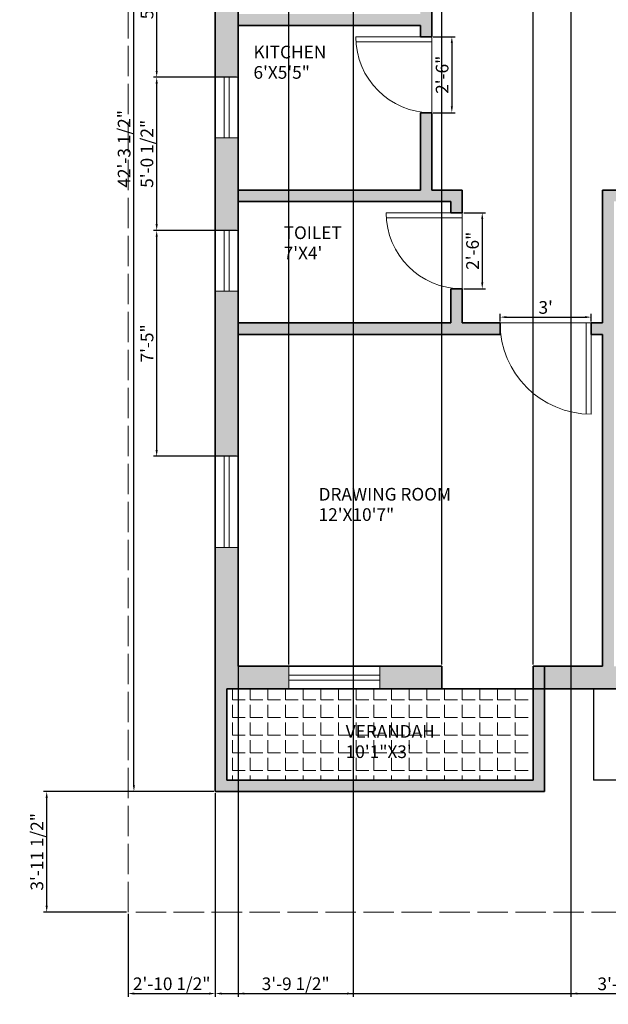
# Model space of a CAD drawing. Units: inches. Extents: x 2871 to 3419, y 1549 to 2228.
# Tile 1 of 3: x 2871 to 3103, y 1549 to 1938. Entities that reach past the tile are written whole.
import ezdxf

# ---------------------------------------------------------------- set-up
doc = ezdxf.new("R2010")
doc.units = ezdxf.units.IN
doc.linetypes.add('ACAD_ISO02W100', pattern=[15, 12, -3])
for name, color, linetype, lineweight in [('A-ANNO-DIMS', 3, 'Continuous', 13), ('A-AREA-IDEN', 3, 'Continuous', 18), ('A-FLOR', 7, 'Continuous', 25), ('A-FLOR-PATT', 30, 'Continuous', 13), ('A-WALL-PATT', 18, 'Continuous', 13), ('C-PROP', 7, 'ACAD_ISO02W100', 18), ('doors', 6, 'Continuous', 18), ('wall', 4, 'Continuous', 35), ('windows', 1, 'Continuous', 18)]:
    doc.layers.add(name, color=color, linetype=linetype, lineweight=lineweight)
doc.styles.get("Standard").update_dxf_attribs({"font": 'arial.ttf', "height": 5})
doc.dimstyles.new('ISO-25', dxfattribs={"dimtxt": 5, "dimasz": 2.5, "dimexe": 1.25, "dimexo": 0.625, "dimtad": 1, "dimlunit": 3, "dimtxsty": 'Standard', "dimcen": 2.5, "dimadec": 0, "dimazin": 0, "dimtfac": 1, "dimtmove": 0, "dimatfit": 3, "dimfxl": 1, "dimarcsym": 0})

# ---------------------------------------------------------------- blocks, each defined once
blk = doc.blocks.new('*D9')
at = {"layer": 'A-ANNO-DIMS', "color": 0, "lineweight": -2, "transparency": 16777216}
for p, q in [((3060.42, 1818.86), (3060.42, 1821.79)), ((3062.92, 1820.54), (3093.92, 1820.54)), ((3096.42, 1818.86), (3096.42, 1821.79))]:
    blk.add_line(p, q, dxfattribs=at)
at = {"layer": 'A-ANNO-DIMS', "color": 0, "transparency": 16777216}
for points in [[(3062.92, 1820.96), (3062.92, 1820.13), (3060.42, 1820.54)], [(3093.92, 1820.96), (3093.92, 1820.13), (3096.42, 1820.54)]]:
    blk.add_solid(points, dxfattribs=at)
at = {"layer": 'Defpoints', "color": 0, "transparency": 16777216}
for p in [(3096.42, 1820.54), (3060.42, 1818.24), (3096.42, 1818.24)]:
    blk.add_point(p, dxfattribs=at)
at = {"layer": 'A-ANNO-DIMS', "color": 0, "transparency": 16777216, "insert": (3078.42, 1823.72), "char_height": 5, "attachment_point": 5}
blk.add_mtext("3'", dxfattribs=at)
blk = doc.blocks.new('*D10')
at = {"layer": 'A-ANNO-DIMS', "color": 0, "lineweight": -2, "transparency": 16777216}
for p, q in [((3046.04, 1861.74), (3054.62, 1861.74)), ((3053.37, 1859.24), (3053.37, 1834.24)), ((3046.04, 1831.74), (3054.62, 1831.74))]:
    blk.add_line(p, q, dxfattribs=at)
at = {"layer": 'A-ANNO-DIMS', "color": 0, "transparency": 16777216}
for points in [[(3052.95, 1859.24), (3053.79, 1859.24), (3053.37, 1861.74)], [(3052.95, 1834.24), (3053.79, 1834.24), (3053.37, 1831.74)]]:
    blk.add_solid(points, dxfattribs=at)
at = {"layer": 'Defpoints', "color": 0, "transparency": 16777216}
for p in [(3045.42, 1861.74), (3045.42, 1831.74), (3053.37, 1831.74)]:
    blk.add_point(p, dxfattribs=at)
at = {"layer": 'A-ANNO-DIMS', "color": 0, "transparency": 16777216, "insert": (3050.19, 1846.74), "char_height": 5, "attachment_point": 5, "rotation": 90}
blk.add_mtext('2\'-6"', dxfattribs=at)
blk = doc.blocks.new('*D11')
at = {"layer": 'A-ANNO-DIMS', "color": 0, "lineweight": -2, "transparency": 16777216}
for p, q in [((3034.04, 1931.24), (3042.61, 1931.24)), ((3041.36, 1928.74), (3041.36, 1903.74)), ((3034.04, 1901.24), (3042.61, 1901.24))]:
    blk.add_line(p, q, dxfattribs=at)
at = {"layer": 'A-ANNO-DIMS', "color": 0, "transparency": 16777216}
for points in [[(3040.94, 1928.74), (3041.77, 1928.74), (3041.36, 1931.24)], [(3040.94, 1903.74), (3041.77, 1903.74), (3041.36, 1901.24)]]:
    blk.add_solid(points, dxfattribs=at)
at = {"layer": 'Defpoints', "color": 0, "transparency": 16777216}
for p in [(3033.42, 1931.24), (3033.42, 1901.24), (3041.36, 1901.24)]:
    blk.add_point(p, dxfattribs=at)
at = {"layer": 'A-ANNO-DIMS', "color": 0, "transparency": 16777216, "insert": (3038.18, 1916.24), "char_height": 5, "attachment_point": 5, "rotation": 90}
blk.add_mtext('2\'-6"', dxfattribs=at)
blk = doc.blocks.new('WIN-36IN')
for p, q in [((0, 36), (0, 0)), ((9, 36), (0, 36)), ((3.5, 0), (3.5, 36)), ((5.5, 0), (5.5, 36)), ((9, 0), (9, 36)), ((0, 0), (9, 0))]:
    blk.add_line(p, q)
blk = doc.blocks.new('WIN-24IN')
for p, q in [((0, 24), (0, 0)), ((9, 24), (0, 24)), ((3.5, 0), (3.5, 24)), ((5.5, 0), (5.5, 24)), ((9, 0), (9, 24)), ((0, 0), (9, 0))]:
    blk.add_line(p, q)
blk = doc.blocks.new('DOOR-SWING-30IN')
for p, q in [((28, 29.93), (28, 0)), ((30, 30), (30, 0)), ((30, 0), (0, 0))]:
    blk.add_line(p, q)
blk.add_arc((30, 0), 30, 90, 180)
blk = doc.blocks.new('DOOR-SWING-36IN')
for p, q in [((0, 36), (0, 0)), ((2, 35.94), (2, 0)), ((0, 0), (36, 0))]:
    blk.add_line(p, q)
blk.add_arc((0, 0), 36, 0, 90)
blk = doc.blocks.new('*D22')
at = {"layer": 'A-ANNO-DIMS', "color": 0, "lineweight": -2, "transparency": 16777216}
for p, q in [((2947.92, 1632.61), (2947.92, 1552.22)), ((3349.42, 1632.61), (3349.42, 1552.22)), ((2950.42, 1553.47), (3346.92, 1553.47))]:
    blk.add_line(p, q, dxfattribs=at)
at = {"layer": 'A-ANNO-DIMS', "color": 0, "transparency": 16777216}
for points in [[(2950.42, 1553.89), (2950.42, 1553.05), (2947.92, 1553.47)], [(3346.92, 1553.89), (3346.92, 1553.05), (3349.42, 1553.47)]]:
    blk.add_solid(points, dxfattribs=at)
at = {"layer": 'Defpoints', "color": 0, "transparency": 16777216}
for p in [(2947.92, 1633.24), (3349.42, 1633.24), (3349.42, 1553.47)]:
    blk.add_point(p, dxfattribs=at)
at = {"layer": 'A-ANNO-DIMS', "color": 0, "transparency": 16777216, "insert": (3148.67, 1556.68), "char_height": 5, "attachment_point": 5}
blk.add_mtext('33\'-5 1/2"', dxfattribs=at)
blk = doc.blocks.new('*D23')
at = {"layer": 'A-ANNO-DIMS', "color": 0, "lineweight": -2, "transparency": 16777216}
for p, q in [((2947.29, 2140.74), (2914.52, 2140.74)), ((2915.77, 1635.74), (2915.77, 2138.24)), ((2947.29, 1633.24), (2914.52, 1633.24))]:
    blk.add_line(p, q, dxfattribs=at)
at = {"layer": 'A-ANNO-DIMS', "color": 0, "transparency": 16777216}
for points in [[(2915.35, 2138.24), (2916.18, 2138.24), (2915.77, 2140.74)], [(2915.35, 1635.74), (2916.18, 1635.74), (2915.77, 1633.24)]]:
    blk.add_solid(points, dxfattribs=at)
at = {"layer": 'Defpoints', "color": 0, "transparency": 16777216}
for p in [(2915.77, 2140.74), (2947.92, 2140.74), (2947.92, 1633.24)]:
    blk.add_point(p, dxfattribs=at)
at = {"layer": 'A-ANNO-DIMS', "color": 0, "transparency": 16777216, "insert": (2912.56, 1886.99), "char_height": 5, "attachment_point": 5, "rotation": 90}
blk.add_mtext('42\'-3 1/2"', dxfattribs=at)
blk = doc.blocks.new('*D24')
at = {"layer": 'A-ANNO-DIMS', "color": 0, "lineweight": -2, "transparency": 16777216}
for p, q in [((2947.92, 1632.61), (2947.92, 1552.22)), ((2913.47, 1585), (2913.47, 1552.22)), ((2915.97, 1553.47), (2945.42, 1553.47))]:
    blk.add_line(p, q, dxfattribs=at)
at = {"layer": 'A-ANNO-DIMS', "color": 0, "transparency": 16777216}
for points in [[(2915.97, 1553.89), (2915.97, 1553.05), (2913.47, 1553.47)], [(2945.42, 1553.89), (2945.42, 1553.05), (2947.92, 1553.47)]]:
    blk.add_solid(points, dxfattribs=at)
at = {"layer": 'Defpoints', "color": 0, "transparency": 16777216}
for p in [(2947.92, 1633.24), (2913.47, 1585.62), (2947.92, 1553.47)]:
    blk.add_point(p, dxfattribs=at)
at = {"layer": 'A-ANNO-DIMS', "color": 0, "transparency": 16777216, "insert": (2930.69, 1556.68), "char_height": 5, "attachment_point": 5}
blk.add_mtext('2\'-10 1/2"', dxfattribs=at)
blk = doc.blocks.new('*D25')
at = {"layer": 'A-ANNO-DIMS', "color": 0, "lineweight": -2, "transparency": 16777216}
for p, q in [((2947.29, 1633.24), (2880.07, 1633.24)), ((2881.32, 1588.12), (2881.32, 1630.74)), ((2912.84, 1585.62), (2880.07, 1585.62))]:
    blk.add_line(p, q, dxfattribs=at)
at = {"layer": 'A-ANNO-DIMS', "color": 0, "transparency": 16777216}
for points in [[(2880.9, 1630.74), (2881.73, 1630.74), (2881.32, 1633.24)], [(2880.9, 1588.12), (2881.73, 1588.12), (2881.32, 1585.62)]]:
    blk.add_solid(points, dxfattribs=at)
at = {"layer": 'Defpoints', "color": 0, "transparency": 16777216}
for p in [(2881.32, 1633.24), (2947.92, 1633.24), (2913.47, 1585.62)]:
    blk.add_point(p, dxfattribs=at)
at = {"layer": 'A-ANNO-DIMS', "color": 0, "transparency": 16777216, "insert": (2878.11, 1609.43), "char_height": 5, "attachment_point": 5, "rotation": 90}
blk.add_mtext('3\'-11 1/2"', dxfattribs=at)
blk = doc.blocks.new('*D26')
at = {"layer": 'A-ANNO-DIMS', "color": 0, "lineweight": -2, "transparency": 16777216}
for p, q in [((2956.92, 2131.11), (2956.92, 1552.22)), ((3002.42, 2131.11), (3002.42, 1552.22)), ((2959.42, 1553.47), (2999.92, 1553.47))]:
    blk.add_line(p, q, dxfattribs=at)
at = {"layer": 'A-ANNO-DIMS', "color": 0, "transparency": 16777216}
for points in [[(2959.42, 1553.89), (2959.42, 1553.05), (2956.92, 1553.47)], [(2999.92, 1553.89), (2999.92, 1553.05), (3002.42, 1553.47)]]:
    blk.add_solid(points, dxfattribs=at)
at = {"layer": 'Defpoints', "color": 0, "transparency": 16777216}
for p in [(2956.92, 2131.74), (3002.42, 2131.74), (3002.42, 1553.47)]:
    blk.add_point(p, dxfattribs=at)
at = {"layer": 'A-ANNO-DIMS', "color": 0, "transparency": 16777216, "insert": (2979.67, 1556.68), "char_height": 5, "attachment_point": 5}
blk.add_mtext('3\'-9 1/2"', dxfattribs=at)
blk = doc.blocks.new('*D27')
at = {"layer": 'A-ANNO-DIMS', "color": 0, "lineweight": -2, "transparency": 16777216}
for p, q in [((3088.42, 2131.11), (3088.42, 1552.22)), ((3124.42, 2131.11), (3124.42, 1552.22)), ((3090.92, 1553.47), (3121.92, 1553.47))]:
    blk.add_line(p, q, dxfattribs=at)
at = {"layer": 'A-ANNO-DIMS', "color": 0, "transparency": 16777216}
for points in [[(3090.92, 1553.89), (3090.92, 1553.05), (3088.42, 1553.47)], [(3121.92, 1553.89), (3121.92, 1553.05), (3124.42, 1553.47)]]:
    blk.add_solid(points, dxfattribs=at)
at = {"layer": 'Defpoints', "color": 0, "transparency": 16777216}
for p in [(3088.42, 2131.74), (3124.42, 2131.74), (3124.42, 1553.47)]:
    blk.add_point(p, dxfattribs=at)
at = {"layer": 'A-ANNO-DIMS', "color": 0, "transparency": 16777216, "insert": (3106.42, 1556.65), "char_height": 5, "attachment_point": 5}
blk.add_mtext('3\'-0"', dxfattribs=at)
blk = doc.blocks.new('*D41')
at = {"layer": 'A-ANNO-DIMS', "color": 0, "lineweight": -2, "transparency": 16777216}
for p, q in [((2956.29, 1976.06), (2923.52, 1976.06)), ((2924.77, 1917.79), (2924.77, 1973.56)), ((2956.29, 1915.29), (2923.52, 1915.29))]:
    blk.add_line(p, q, dxfattribs=at)
at = {"layer": 'A-ANNO-DIMS', "color": 0, "transparency": 16777216}
for points in [[(2924.35, 1973.56), (2925.18, 1973.56), (2924.77, 1976.06)], [(2924.35, 1917.79), (2925.18, 1917.79), (2924.77, 1915.29)]]:
    blk.add_solid(points, dxfattribs=at)
at = {"layer": 'Defpoints', "color": 0, "transparency": 16777216}
for p in [(2924.77, 1976.06), (2956.92, 1976.06), (2956.92, 1915.29)]:
    blk.add_point(p, dxfattribs=at)
at = {"layer": 'A-ANNO-DIMS', "color": 0, "transparency": 16777216, "insert": (2921.59, 1945.68), "char_height": 5, "attachment_point": 5, "rotation": 90}
blk.add_mtext('5\'-1"', dxfattribs=at)
blk = doc.blocks.new('*D42')
at = {"layer": 'A-ANNO-DIMS', "color": 0, "lineweight": -2, "transparency": 16777216}
for p, q in [((2956.29, 1915.29), (2923.52, 1915.29)), ((2924.77, 1857.27), (2924.77, 1912.79)), ((2956.29, 1854.77), (2923.52, 1854.77))]:
    blk.add_line(p, q, dxfattribs=at)
at = {"layer": 'A-ANNO-DIMS', "color": 0, "transparency": 16777216}
for points in [[(2924.35, 1912.79), (2925.18, 1912.79), (2924.77, 1915.29)], [(2924.35, 1857.27), (2925.18, 1857.27), (2924.77, 1854.77)]]:
    blk.add_solid(points, dxfattribs=at)
at = {"layer": 'Defpoints', "color": 0, "transparency": 16777216}
for p in [(2924.77, 1915.29), (2956.92, 1915.29), (2956.92, 1854.77)]:
    blk.add_point(p, dxfattribs=at)
at = {"layer": 'A-ANNO-DIMS', "color": 0, "transparency": 16777216, "insert": (2921.56, 1885.03), "char_height": 5, "attachment_point": 5, "rotation": 90}
blk.add_mtext('5\'-0 1/2"', dxfattribs=at)
blk = doc.blocks.new('*D43')
at = {"layer": 'A-ANNO-DIMS', "color": 0, "lineweight": -2, "transparency": 16777216}
for p, q in [((2956.29, 1854.77), (2923.52, 1854.77)), ((2924.77, 1768.09), (2924.77, 1852.27)), ((2956.29, 1765.59), (2923.52, 1765.59))]:
    blk.add_line(p, q, dxfattribs=at)
at = {"layer": 'A-ANNO-DIMS', "color": 0, "transparency": 16777216}
for points in [[(2924.35, 1852.27), (2925.18, 1852.27), (2924.77, 1854.77)], [(2924.35, 1768.09), (2925.18, 1768.09), (2924.77, 1765.59)]]:
    blk.add_solid(points, dxfattribs=at)
at = {"layer": 'Defpoints', "color": 0, "transparency": 16777216}
for p in [(2924.77, 1854.77), (2956.92, 1854.77), (2956.92, 1765.59)]:
    blk.add_point(p, dxfattribs=at)
at = {"layer": 'A-ANNO-DIMS', "color": 0, "transparency": 16777216, "insert": (2921.6, 1810.18), "char_height": 5, "attachment_point": 5, "rotation": 90}
blk.add_mtext('7\'-5"', dxfattribs=at)
blk = doc.blocks.new('*D44')
at = {"layer": 'A-ANNO-DIMS', "color": 0, "lineweight": -2, "transparency": 16777216}
for p, q in [((2956.92, 1683.36), (2956.92, 2219.02)), ((2959.42, 2217.77), (2974.42, 2217.77)), ((2976.92, 1683.36), (2976.92, 2219.02))]:
    blk.add_line(p, q, dxfattribs=at)
at = {"layer": 'A-ANNO-DIMS', "color": 0, "transparency": 16777216}
for points in [[(2959.42, 2218.19), (2959.42, 2217.35), (2956.92, 2217.77)], [(2974.42, 2218.19), (2974.42, 2217.35), (2976.92, 2217.77)]]:
    blk.add_solid(points, dxfattribs=at)
at = {"layer": 'Defpoints', "color": 0, "transparency": 16777216}
for p in [(2976.92, 2217.77), (2956.92, 1682.74), (2976.92, 1682.74)]:
    blk.add_point(p, dxfattribs=at)
at = {"layer": 'A-ANNO-DIMS', "color": 0, "transparency": 16777216, "insert": (2966.92, 2220.95), "char_height": 5, "attachment_point": 5}
blk.add_mtext('1\'-8"', dxfattribs=at)
blk = doc.blocks.new('*D46')
at = {"layer": 'A-ANNO-DIMS', "color": 0, "lineweight": -2, "transparency": 16777216}
for p, q in [((3037.42, 1683.36), (3037.42, 2219.02)), ((3039.92, 2217.77), (3070.92, 2217.77)), ((3073.42, 1683.36), (3073.42, 2219.02))]:
    blk.add_line(p, q, dxfattribs=at)
at = {"layer": 'A-ANNO-DIMS', "color": 0, "transparency": 16777216}
for points in [[(3039.92, 2218.19), (3039.92, 2217.35), (3037.42, 2217.77)], [(3070.92, 2218.19), (3070.92, 2217.35), (3073.42, 2217.77)]]:
    blk.add_solid(points, dxfattribs=at)
at = {"layer": 'Defpoints', "color": 0, "transparency": 16777216}
for p in [(3073.42, 2217.77), (3037.42, 1682.74), (3073.42, 1682.74)]:
    blk.add_point(p, dxfattribs=at)
at = {"layer": 'A-ANNO-DIMS', "color": 0, "transparency": 16777216, "insert": (3055.42, 2220.95), "char_height": 5, "attachment_point": 5}
blk.add_mtext('3\'-0"', dxfattribs=at)
blk = doc.blocks.new('*D48')
at = {"layer": 'A-ANNO-DIMS', "color": 0, "lineweight": -2, "transparency": 16777216}
for p, q in [((2976.92, 1683.36), (2976.92, 2219.02)), ((2979.42, 2217.77), (3034.92, 2217.77)), ((3037.42, 1683.36), (3037.42, 2219.02))]:
    blk.add_line(p, q, dxfattribs=at)
at = {"layer": 'A-ANNO-DIMS', "color": 0, "transparency": 16777216}
for points in [[(2979.42, 2218.19), (2979.42, 2217.35), (2976.92, 2217.77)], [(3034.92, 2218.19), (3034.92, 2217.35), (3037.42, 2217.77)]]:
    blk.add_solid(points, dxfattribs=at)
at = {"layer": 'Defpoints', "color": 0, "transparency": 16777216}
for p in [(3037.42, 2217.77), (2976.92, 1682.74), (3037.42, 1682.74)]:
    blk.add_point(p, dxfattribs=at)
at = {"layer": 'A-ANNO-DIMS', "color": 0, "transparency": 16777216, "insert": (3007.17, 2220.98), "char_height": 5, "attachment_point": 5}
blk.add_mtext('5\'-0 1/2"', dxfattribs=at)

msp = doc.modelspace()

# ---------------------------------------------------------------- hatches: boundary and pattern name
at = {"layer": 'A-FLOR-PATT'}
h = msp.add_hatch(dxfattribs=at)
h.set_pattern_fill('ANGLE', color=256)
h.set_pattern_definition([(0, (0, 0), (0, 6.985), [5.08, -1.905]), (90, (0, 0), (-6.985, 4e-16), [5.08, -1.905])])
h.paths.add_polyline_path([(3073.418, 1673.735), (3037.418, 1673.735), (2952.418, 1673.735), (2952.418, 1637.735), (3073.418, 1637.735)])
h.paths.add_polyline_path([(3344.918, 1673.735), (3259.918, 1673.735), (3223.918, 1673.735), (3223.918, 1637.735), (3344.918, 1637.735)])
h.paths.add_polyline_path([(2998.155, 1645.095), (3026.055, 1645.095), (3026.055, 1652.758), (2998.155, 1652.758)], flags=24)
h.paths.add_polyline_path([(2998.183, 1653.243), (3039.496, 1653.243), (3039.496, 1660.743), (2998.183, 1660.743)], flags=24)
h.paths.add_polyline_path([(3263.884, 1645.095), (3291.783, 1645.095), (3291.783, 1652.758), (3263.884, 1652.758)], flags=24)
h.paths.add_polyline_path([(3263.911, 1653.243), (3305.224, 1653.243), (3305.224, 1660.743), (3263.911, 1660.743)], flags=24)
at = {"layer": 'A-WALL-PATT'}
h = msp.add_hatch(color=256, dxfattribs=at)
h.dxf.hatch_style = 1
h.paths.add_polyline_path([(2956.918, 2131.735), (3002.418, 2131.735), (3002.418, 2140.735), (2947.918, 2140.735), (2947.918, 2079.154), (2956.918, 2079.154)])
h.paths.add_polyline_path([(3252.668, 2140.735), (3160.418, 2140.735), (3160.418, 2131.735), (3196.418, 2131.735), (3196.418, 1992.735), (3128.918, 1992.735), (3128.918, 1988.235), (3160.418, 1988.235), (3160.418, 1870.735), (3160.418, 1866.235), (3164.918, 1866.235), (3164.918, 1890.235), (3164.918, 1988.235), (3205.418, 1988.235), (3205.418, 1992.735), (3200.918, 1992.735), (3200.918, 2131.735), (3252.668, 2131.735)])
h.paths.add_polyline_path([(3349.418, 2140.735), (3288.668, 2140.735), (3288.668, 2131.735), (3340.418, 2131.735), (3340.418, 2080.235), (3349.418, 2080.235)])
h.paths.add_polyline_path([(3349.418, 2044.235), (3340.418, 2044.235), (3340.418, 1992.735), (3302.918, 1992.735), (3302.918, 1988.235), (3340.418, 1988.235), (3340.418, 1976.235), (3349.418, 1976.235)])
h.paths.add_polyline_path([(3349.418, 1952.235), (3340.418, 1952.235), (3340.418, 1940.235), (3268.418, 1940.235), (3268.418, 1988.235), (3272.918, 1988.235), (3272.918, 1992.735), (3241.418, 1992.735), (3241.418, 1988.235), (3263.918, 1988.235), (3263.918, 1931.235), (3268.418, 1931.235), (3268.418, 1935.735), (3340.418, 1935.735), (3340.418, 1915.235), (3349.418, 1915.235)])
h.paths.add_polyline_path([(3349.418, 1891.235), (3340.418, 1891.235), (3340.418, 1870.735), (3268.418, 1870.735), (3268.418, 1901.235), (3263.918, 1901.235), (3263.918, 1870.735), (3251.918, 1870.735), (3251.918, 1866.235), (3251.918, 1861.735), (3256.418, 1861.735), (3256.418, 1866.235), (3340.418, 1866.235), (3340.418, 1854.235), (3349.418, 1854.235)])
h.paths.add_polyline_path([(3349.418, 1830.235), (3340.418, 1830.235), (3340.418, 1818.235), (3256.418, 1818.235), (3256.418, 1831.735), (3251.918, 1831.735), (3251.918, 1818.235), (3236.918, 1818.235), (3236.918, 1813.735), (3340.418, 1813.735), (3340.418, 1766.452), (3349.418, 1766.452)])
h.paths.add_polyline_path([(3349.418, 1730.452), (3340.418, 1730.452), (3340.418, 1682.735), (3320.418, 1682.735), (3320.418, 1673.735), (3344.918, 1673.735), (3344.918, 1637.735), (3223.918, 1637.735), (3223.918, 1673.735), (3219.418, 1673.735), (3219.418, 1633.235), (3349.418, 1633.235)])
h.paths.add_polyline_path([(3284.418, 1682.735), (3259.918, 1682.735), (3259.918, 1673.735), (3284.418, 1673.735)], flags=17)
h.paths.add_polyline_path([(3223.918, 1682.735), (3219.418, 1682.735), (3219.418, 1673.735), (3223.918, 1673.735)], flags=17)
h.paths.add_polyline_path([(3196.418, 1813.735), (3200.918, 1813.735), (3200.918, 1818.235), (3196.418, 1818.235), (3196.418, 1866.235), (3196.418, 1870.735), (3188.918, 1870.735), (3188.918, 1866.235), (3191.918, 1866.235), (3191.918, 1682.735), (3160.668, 1682.735), (3160.668, 1673.735), (3219.418, 1673.735), (3219.418, 1682.735), (3196.418, 1682.735)])
h.paths.add_polyline_path([(3105.418, 1866.235), (3130.418, 1866.235), (3130.418, 1870.735), (3100.918, 1870.735), (3100.918, 1866.235), (3100.918, 1818.235), (3096.418, 1818.235), (3096.418, 1813.735), (3100.918, 1813.735), (3100.918, 1682.735), (3077.918, 1682.735), (3077.918, 1673.735), (3136.668, 1673.735), (3136.668, 1682.735), (3105.418, 1682.735)])
h.paths.add_polyline_path([(3077.918, 1682.735), (3073.418, 1682.735), (3073.418, 1673.735), (3077.918, 1673.735)], flags=17)
h.paths.add_polyline_path([(3077.918, 1673.735), (3073.418, 1673.735), (3073.418, 1637.735), (2952.418, 1637.735), (2952.418, 1673.735), (2976.918, 1673.735), (2976.918, 1682.735), (2956.918, 1682.735), (2956.918, 1729.593), (2947.918, 1729.593), (2947.918, 1633.235), (3077.918, 1633.235)])
h.paths.add_polyline_path([(3037.418, 1682.735), (3012.918, 1682.735), (3012.918, 1673.735), (3037.418, 1673.735)], flags=17)
h.paths.add_polyline_path([(3060.418, 1818.235), (3045.418, 1818.235), (3045.418, 1831.735), (3040.918, 1831.735), (3040.918, 1818.235), (2956.918, 1818.235), (2956.918, 1830.772), (2947.918, 1830.772), (2947.918, 1765.593), (2956.918, 1765.593), (2956.918, 1813.735), (3060.418, 1813.735)])
h.paths.add_polyline_path([(3045.418, 1870.735), (3033.418, 1870.735), (3033.418, 1901.235), (3028.918, 1901.235), (3028.918, 1870.735), (2956.918, 1870.735), (2956.918, 1891.289), (2947.918, 1891.289), (2947.918, 1854.772), (2956.918, 1854.772), (2956.918, 1866.235), (3040.918, 1866.235), (3040.918, 1861.735), (3045.418, 1861.735), (3045.418, 1866.235)])
h.paths.add_polyline_path([(3033.418, 1988.235), (3043.418, 1988.235), (3043.418, 1992.735), (3024.418, 1992.735), (3024.418, 1988.235), (3028.918, 1988.235), (3028.918, 1940.235), (2956.918, 1940.235), (2956.918, 1952.063), (2947.918, 1952.063), (2947.918, 1915.289), (2956.918, 1915.289), (2956.918, 1935.735), (3028.918, 1935.735), (3028.918, 1931.235), (3033.418, 1931.235)])
h.paths.add_polyline_path([(2956.918, 2043.154), (2947.918, 2043.154), (2947.918, 1976.063), (2956.918, 1976.063), (2956.918, 1988.235), (2994.418, 1988.235), (2994.418, 1992.735), (2956.918, 1992.735)])

# ---------------------------------------------------------------- linework, layer by layer
at = {"layer": 'A-FLOR'}
for p in [(3097.318, 1673.735), (3200.352, 1637.735)]:
    msp.add_line(p, (3097.318, 1637.735), dxfattribs=at)
at = {"layer": 'C-PROP'}
for p, q in [((2913.468, 1585.622), (2913.468, 2185.622)), ((3393.468, 1585.622), (2913.468, 1585.622))]:
    msp.add_line(p, q, dxfattribs=at)
at = {"layer": 'wall'}
for p, q in [((2947.918, 2140.735), (2947.918, 1633.235)), ((3033.418, 1988.235), (3033.418, 1931.235)), ((3028.918, 1935.735), (2956.918, 1935.735)), ((2956.918, 1935.735), (2956.918, 1870.735)), ((3028.918, 1935.735), (3028.918, 1931.235)), ((3028.918, 1931.235), (3033.418, 1931.235)), ((3028.918, 1901.235), (3033.418, 1901.235)), ((3028.918, 1901.235), (3028.918, 1870.735)), ((3033.418, 1901.235), (3033.418, 1870.735)), ((3028.918, 1870.735), (2956.918, 1870.735)), ((3045.418, 1870.735), (3033.418, 1870.735)), ((3045.418, 1866.235), (3045.418, 1870.735)), ((3100.918, 1866.235), (3100.918, 1870.735)), ((3130.418, 1870.735), (3100.918, 1870.735)), ((2956.918, 1866.235), (2956.918, 1818.235)), ((3040.918, 1866.235), (2956.918, 1866.235)), ((3040.918, 1866.235), (3040.918, 1861.735)), ((3045.418, 1866.235), (3045.418, 1861.735)), ((3100.918, 1866.235), (3100.918, 1818.235)), ((3040.918, 1861.735), (3045.418, 1861.735)), ((3040.918, 1831.735), (3045.418, 1831.735)), ((3040.918, 1831.735), (3040.918, 1818.235)), ((3045.418, 1831.735), (3045.418, 1818.235)), ((3040.918, 1818.235), (2956.918, 1818.235)), ((3060.418, 1818.235), (3045.418, 1818.235)), ((3060.418, 1813.735), (3060.418, 1818.235)), ((3100.918, 1818.235), (3096.418, 1818.235)), ((3096.418, 1813.735), (3096.418, 1818.235)), ((2956.918, 1813.735), (2956.918, 1682.735)), ((3060.418, 1813.735), (2956.918, 1813.735)), ((3100.918, 1813.735), (3096.418, 1813.735)), ((3100.918, 1813.735), (3100.918, 1682.735)), ((3037.418, 1682.735), (2956.918, 1682.735)), ((3037.418, 1673.735), (3037.418, 1682.735)), ((3100.918, 1682.735), (3073.418, 1682.735)), ((3073.418, 1673.735), (3073.418, 1682.735)), ((3077.918, 1682.735), (3077.918, 1633.235)), ((2952.418, 1673.735), (2952.418, 1637.735)), ((3037.418, 1673.735), (2952.418, 1673.735)), ((3037.418, 1673.735), (3073.418, 1673.735)), ((3073.418, 1673.735), (3073.418, 1637.735)), ((3223.918, 1673.735), (3073.418, 1673.735)), ((3073.418, 1637.735), (2952.418, 1637.735)), ((3077.918, 1633.235), (2947.918, 1633.235))]:
    msp.add_line(p, q, dxfattribs=at)

# ---------------------------------------------------------------- block references
at = {"layer": 'doors'}
for name, p, rotation in [('DOOR-SWING-30IN', (3033.418, 1901.235), 89.99999999999883), ('DOOR-SWING-30IN', (3045.418, 1831.735), 89.99999999999883), ('DOOR-SWING-36IN', (3096.419, 1818.235), 180)]:
    msp.add_blockref(name, p, dxfattribs=dict(at, rotation=rotation))
at = {"layer": 'windows'}
for p in [(2947.918, 1891.289), (2947.918, 1830.772)]:
    msp.add_blockref('WIN-24IN', p, dxfattribs=at)
for p, rotation in [((2956.919, 1765.594), 180), ((2976.918, 1682.735), 269.999999999999)]:
    msp.add_blockref('WIN-36IN', p, dxfattribs=dict(at, rotation=rotation))

# ---------------------------------------------------------------- texts
at = {"layer": 'A-AREA-IDEN'}
for s, p in [('KITCHEN', (2962.999, 1922.702)), ('6\'X5\'5"', (2962.999, 1914.67)), ('TOILET', (2974.93, 1851.375)), ("7'X4'", (2974.93, 1843.343)), ('DRAWING ROOM', (2988.729, 1748.118)), ('12\'X10\'7"', (2988.729, 1740.086)), ('VERANDAH', (2999.433, 1654.493)), ('10\'1"X3\'', (2999.433, 1646.461))]:
    msp.add_text(s, height=5, dxfattribs=at).set_placement(p)

# ---------------------------------------------------------------- dimensions: what is measured, and where the dimension line sits
at = {"layer": 'A-ANNO-DIMS'}
for base, p1, p2, override, picture, middle in [((3037.418, 2217.772), (2976.918, 1682.735), (3037.418, 1682.735), {"dimdec": 1, "dimlfac": 1, "dimrnd": 0, "dimzin": 1, "dimdsep": 46, "dimlunit": 4, "dimfrac": 2}, '*D48', (3007.168, 2220.982)), ((2976.918, 2217.772), (2956.918, 1682.735), (2976.918, 1682.735), {"dimdec": 1, "dimlfac": 1, "dimrnd": 0, "dimzin": 1, "dimdsep": 46, "dimlunit": 4, "dimfrac": 2}, '*D44', (2966.918, 2220.949)), ((3073.418, 2217.772), (3037.418, 1682.735), (3073.418, 1682.735), {"dimdec": 1, "dimlfac": 1, "dimrnd": 0, "dimzin": 1, "dimdsep": 46, "dimlunit": 4, "dimfrac": 2}, '*D46', (3055.418, 2220.951)), ((3002.418, 1553.472), (2956.918, 2131.735), (3002.418, 2131.735), {"dimdec": 1, "dimlfac": 1, "dimrnd": 0, "dimzin": 1, "dimdsep": 46, "dimlunit": 4, "dimfrac": 2}, '*D26', (2979.668, 1556.683)), ((3124.418, 1553.472), (3088.418, 2131.735), (3124.418, 2131.735), {"dimdec": 1, "dimlfac": 1, "dimrnd": 0, "dimzin": 1, "dimdsep": 46, "dimlunit": 4, "dimfrac": 2}, '*D27', (3106.418, 1556.651)), ((3096.418, 1820.544), (3060.418, 1818.235), (3096.418, 1818.235), {"dimclrd": 0, "dimclre": 0, "dimclrt": 0}, '*D9', (3078.418, 1823.724)), ((2947.9183, 1553.4715), (2913.4677, 1585.6215), (2947.9183, 1633.2351), {"dimdec": 1, "dimlfac": 1, "dimrnd": 0, "dimzin": 1, "dimdsep": 46, "dimlunit": 4, "dimfrac": 2}, '*D24', (2930.693, 1556.6818)), ((3349.418, 1553.472), (2947.918, 1633.235), (3349.418, 1633.235), {"dimdec": 1, "dimlfac": 1, "dimrnd": 0, "dimzin": 1, "dimdsep": 46, "dimlunit": 4, "dimfrac": 2}, '*D22', (3148.668, 1556.683))]:
    dim = msp.add_linear_dim(base=base, p1=p1, p2=p2, dimstyle='ISO-25', override=override, dxfattribs=at)
    dim.commit()
    dim.dimension.update_dxf_attribs({"geometry": picture, "text_midpoint": middle})
for base, p1, p2, override, picture, middle in [((2915.768, 2140.735), (2947.918, 1633.235), (2947.918, 2140.735), {"dimdec": 1, "dimlfac": 1, "dimrnd": 0, "dimzin": 1, "dimdsep": 46, "dimlunit": 4, "dimfrac": 2}, '*D23', (2912.556, 1886.985)), ((2924.768, 1976.063), (2956.918, 1915.289), (2956.918, 1976.063), {"dimdec": 1, "dimlfac": 1, "dimrnd": 0, "dimzin": 1, "dimdsep": 46, "dimlunit": 4, "dimfrac": 2}, '*D41', (2921.59, 1945.676)), ((3041.357, 1901.235), (3033.418, 1931.235), (3033.418, 1901.235), {"dimclrd": 0, "dimclre": 0, "dimclrt": 0}, '*D11', (3038.18, 1916.235)), ((2924.768, 1915.289), (2956.918, 1854.772), (2956.918, 1915.289), {"dimdec": 1, "dimlfac": 1, "dimrnd": 0, "dimzin": 1, "dimdsep": 46, "dimlunit": 4, "dimfrac": 2}, '*D42', (2921.558, 1885.031)), ((3053.369, 1831.735), (3045.418, 1861.735), (3045.418, 1831.735), {"dimclrd": 0, "dimclre": 0, "dimclrt": 0}, '*D10', (3050.191, 1846.735)), ((2924.768, 1854.772), (2956.918, 1765.593), (2956.918, 1854.772), {"dimdec": 1, "dimlfac": 1, "dimrnd": 0, "dimzin": 1, "dimdsep": 46, "dimlunit": 4, "dimfrac": 2}, '*D43', (2921.601, 1810.183)), ((2881.318, 1633.235), (2913.468, 1585.622), (2947.918, 1633.235), {"dimdec": 1, "dimlfac": 1, "dimrnd": 0, "dimzin": 1, "dimdsep": 46, "dimlunit": 4, "dimfrac": 2}, '*D25', (2878.106, 1609.428))]:
    dim = msp.add_linear_dim(base=base, p1=p1, p2=p2, angle=90, dimstyle='ISO-25', override=override, dxfattribs=at)
    dim.commit()
    dim.dimension.update_dxf_attribs({"geometry": picture, "text_midpoint": middle})

doc.saveas('drawing.dxf')
